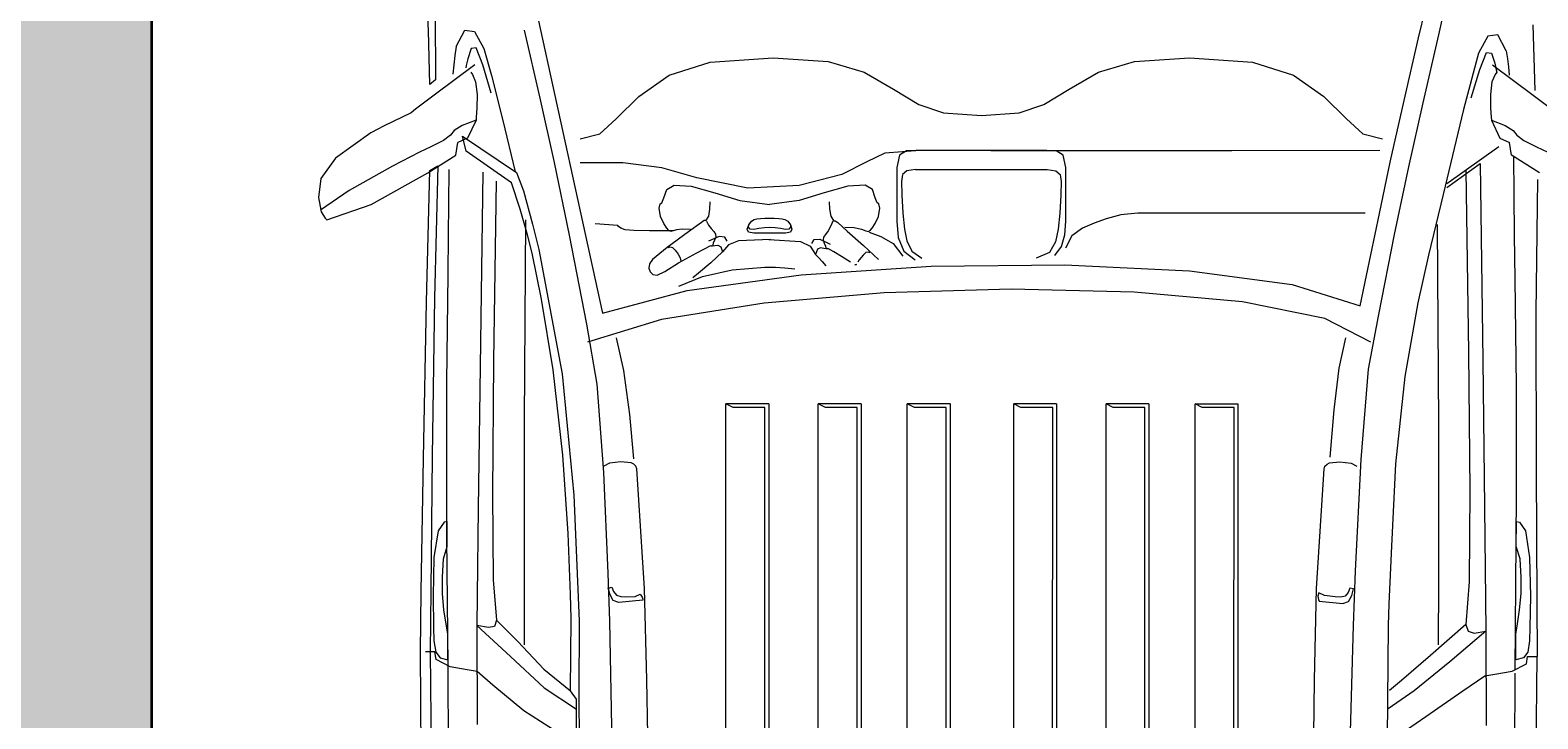
# Model space of a CAD drawing. Units: inches. Extents: x -16 to 587, y -783 to 64.
# Tile 4 of 14: x 111 to 195, y -633 to -595. Entities that reach past the tile are written whole.
import ezdxf

# ---------------------------------------------------------------- set-up
doc = ezdxf.new("R2010")
doc.units = ezdxf.units.IN
doc.header["$MEASUREMENT"] = 0
for name, color, linetype, lineweight in [('A-ANNO-DIMS', 2, 'Continuous', 18), ('A-SITE-VEHC', 8, 'Continuous', 13), ('A-WALL', 7, 'Continuous', 35), ('A-WALL-PATT', 23, 'Continuous', 13)]:
    doc.layers.add(name, color=color, linetype=linetype, lineweight=lineweight)
doc.styles.get("Standard").update_dxf_attribs({"font": 'arial.ttf'})
doc.dimstyles.get("Standard").update_dxf_attribs({"dimtxt": 0.18, "dimasz": 0.18, "dimexe": 0.18, "dimexo": 0.0625, "dimgap": 0.09, "dimtad": 0, "dimtih": 1, "dimtoh": 1, "dimdec": 0, "dimzin": 0, "dimdsep": 46, "dimlunit": 3, "dimtxsty": 'Standard', "dimcen": 0.09, "dimadec": 0, "dimazin": 0, "dimtfac": 1, "dimtdec": 0, "dimtofl": 0, "dimtmove": 0, "dimatfit": 3, "dimfxl": 1, "dimtolj": 1, "dimtzin": 0, "dimarcsym": 0})

# ---------------------------------------------------------------- blocks, each defined once
blk = doc.blocks.new('*D56')
at = {"layer": 'A-ANNO-DIMS', "color": 0, "lineweight": -2, "transparency": 16777216}
for p, q in [((118.083, -728.492), (118.083, 63.775)), ((228.083, -728.492), (228.083, 63.775)), ((118.263, 63.595), (172.753, 63.595)), ((227.903, 63.595), (173.412, 63.595))]:
    blk.add_line(p, q, dxfattribs=at)
at = {"layer": 'A-ANNO-DIMS', "color": 0, "transparency": 16777216}
for points in [[(118.263, 63.625), (118.263, 63.565), (118.083, 63.595)], [(227.903, 63.625), (227.903, 63.565), (228.083, 63.595)]]:
    blk.add_solid(points, dxfattribs=at)
at = {"layer": 'Defpoints', "color": 0, "transparency": 16777216}
for p in [(228.083, 63.595), (118.083, -728.555), (228.083, -728.555)]:
    blk.add_point(p, dxfattribs=at)
at = {"layer": 'A-ANNO-DIMS', "color": 0, "transparency": 16777216, "insert": (173.083, 63.595), "char_height": 0.18, "attachment_point": 5}
blk.add_mtext('\\A1;9\'-2"', dxfattribs=at)

msp = doc.modelspace()

# ---------------------------------------------------------------- hatches: boundary and pattern name
at = {"layer": 'A-WALL-PATT'}
h = msp.add_hatch(color=256, dxfattribs=at)
h.dxf.hatch_style = 1
h.paths.add_polyline_path([(137.083, -543.555), (137.083, -534.555), (118.083, -534.555), (118.083, -528.555), (109.083, -528.555), (109.083, -534.555), (109.083, -672.555), (118.083, -672.555), (118.083, -543.555)], flags=17)
h.paths.add_polyline_path([(27.083, -663.555), (27.083, -400.555), (73.083, -400.555), (73.083, -391.555), (27.083, -391.555), (27.083, 10.445), (48.751, 10.445), (171.083, 10.445), (171.083, -17.555), (180.083, -17.555), (180.083, 10.445), (228.083, 10.445), (228.083, -262.555), (206.414, -262.555), (118.083, -262.555), (118.083, -271.555), (228.083, -271.555), (228.083, -391.555), (154.083, -391.555), (154.083, -400.555), (228.083, -400.555), (228.083, -534.555), (209.083, -534.555), (209.083, -543.555), (237.083, -543.555), (237.083, 19.445), (18.083, 19.445), (18.083, -672.555), (73.083, -672.555), (73.083, -663.555)])
h.paths.add_polyline_path([(109.083, -486.555), (87.083, -486.555), (87.083, -495.555), (118.083, -495.555), (118.083, -400.555), (118.083, -391.555), (109.083, -391.555), (109.083, -400.555)], flags=17)

# ---------------------------------------------------------------- linework, layer by layer
at = {"layer": 'A-SITE-VEHC'}
for p, q in [((133.461, -595.126), (133.365, -593.07)), ((139.402, -593.833), (143.123, -610.827)), ((189.973, -593.605), (189.568, -595.361)), ((133.831, -594.204), (133.86, -597.859)), ((188.472, -595.539), (188.846, -593.942)), ((133.539, -598.134), (133.461, -595.126)), ((135.003, -596.012), (135.48, -595.11)), ((135.48, -595.11), (136.023, -595.18)), ((136.023, -595.18), (136.539, -596.13)), ((138.777, -595.108), (139.641, -598.886)), ((187.665, -599.023), (188.472, -595.539)), ((189.568, -595.361), (188.703, -599.139)), ((192.321, -595.433), (191.805, -596.383)), ((192.864, -595.363), (192.321, -595.433)), ((193.341, -596.265), (192.864, -595.363)), ((194.817, -594.806), (194.93, -598.464)), ((135.003, -596.012), (134.931, -596.516)), ((135.83, -596.13), (135.648, -596.695)), ((136.108, -596.091), (135.83, -596.13)), ((136.478, -597.036), (136.108, -596.091)), ((136.539, -596.13), (136.965, -597.635)), ((191.805, -596.383), (190.967, -599.517)), ((191.866, -597.289), (192.236, -596.343)), ((192.236, -596.343), (192.514, -596.383)), ((192.514, -596.383), (192.696, -596.948)), ((193.341, -596.265), (193.404, -596.702)), ((136.045, -597.033), (133.786, -598.721)), ((134.869, -597.03), (134.815, -597.554)), ((134.931, -596.516), (134.869, -597.03)), ((135.559, -597.063), (135.535, -597.194)), ((135.648, -596.695), (135.559, -597.063)), ((136.953, -598.612), (136.478, -597.036)), ((146.838, -597.613), (149.114, -596.892)), ((149.114, -596.892), (152.61, -596.647)), ((152.61, -596.647), (155.674, -596.854)), ((155.674, -596.854), (157.672, -597.445)), ((170.682, -597.445), (172.679, -596.854)), ((172.679, -596.854), (175.744, -596.647)), ((175.744, -596.647), (179.24, -596.892)), ((179.24, -596.892), (181.516, -597.613)), ((192.573, -597.033), (194.832, -598.721)), ((192.696, -596.948), (192.785, -597.315)), ((193.404, -596.702), (193.46, -597.147)), ((193.46, -597.147), (193.509, -597.6)), ((133.86, -597.859), (133.539, -598.134)), ((135.809, -597.447), (135.901, -597.571)), ((135.901, -597.571), (136.071, -597.972)), ((136.071, -597.972), (136.163, -598.688)), ((136.965, -597.635), (137.589, -600.122)), ((145.147, -598.791), (146.838, -597.613)), ((157.672, -597.445), (159.298, -598.38)), ((169.056, -598.38), (170.682, -597.445)), ((181.516, -597.613), (183.207, -598.791)), ((191.391, -598.865), (191.866, -597.289)), ((192.547, -597.972), (192.455, -598.688)), ((192.718, -597.571), (192.547, -597.972)), ((192.809, -597.447), (192.718, -597.571)), ((192.785, -597.315), (192.809, -597.447)), ((133.786, -598.721), (132.748, -599.502)), ((136.163, -598.688), (136.148, -599.449)), ((139.641, -598.886), (140.44, -602.454)), ((143.891, -600.03), (145.147, -598.791)), ((159.298, -598.38), (160.705, -599.245)), ((167.649, -599.245), (169.056, -598.38)), ((183.207, -598.791), (184.463, -600.03)), ((192.455, -598.688), (192.47, -599.449)), ((194.832, -598.721), (195.87, -599.502)), ((132.499, -599.693), (131.998, -599.935)), ((132.748, -599.502), (132.499, -599.693)), ((136.148, -599.449), (136.12, -599.935)), ((160.705, -599.245), (162.081, -599.704)), ((162.081, -599.704), (164.177, -599.84)), ((164.177, -599.84), (166.273, -599.704)), ((166.273, -599.704), (167.649, -599.245)), ((186.897, -602.432), (187.665, -599.023)), ((188.703, -599.139), (187.904, -602.707)), ((190.967, -599.517), (189.826, -604.241)), ((192.47, -599.449), (192.499, -599.935)), ((130.998, -600.427), (130.253, -600.815)), ((131.998, -599.935), (130.998, -600.427)), ((135.342, -600.4), (134.896, -600.68)), ((136.104, -600.106), (135.342, -600.4)), ((136.104, -600.106), (135.631, -601.111)), ((136.12, -599.935), (136.104, -600.106)), ((137.589, -600.122), (138.277, -602.975)), ((142.987, -600.86), (143.891, -600.03)), ((184.463, -600.03), (185.367, -600.86)), ((192.499, -599.935), (192.514, -600.106)), ((192.514, -600.106), (192.987, -601.111)), ((192.514, -600.106), (193.276, -600.4)), ((193.276, -600.4), (193.722, -600.68)), ((130.253, -600.815), (128.305, -602.219)), ((134.294, -601.231), (133.6, -601.582)), ((134.686, -600.934), (134.294, -601.231)), ((134.896, -600.68), (134.686, -600.934)), ((134.981, -602.057), (135.099, -601.347)), ((135.631, -601.111), (135.099, -601.347)), ((135.348, -600.995), (138.346, -603.01)), ((135.554, -601.82), (135.348, -600.995)), ((141.894, -601.147), (142.987, -600.86)), ((185.367, -600.86), (186.46, -601.147)), ((192.987, -601.111), (193.519, -601.347)), ((193.637, -602.057), (193.519, -601.347)), ((193.722, -600.68), (193.932, -600.934)), ((193.932, -600.934), (194.324, -601.231)), ((194.324, -601.231), (195.018, -601.582)), ((128.305, -602.219), (127.485, -603.354)), ((132.972, -601.879), (131.466, -602.664)), ((133.6, -601.582), (132.972, -601.879)), ((133.428, -603.026), (134.981, -602.057)), ((138.071, -603.582), (135.554, -601.82)), ((158.816, -601.944), (157.813, -602.417)), ((160.78, -601.785), (158.816, -601.944)), ((159.628, -602.053), (159.48, -602.729)), ((160.012, -601.816), (159.628, -602.053)), ((160.544, -601.787), (160.012, -601.816)), ((167.81, -601.787), (160.544, -601.787)), ((164.711, -601.806), (160.78, -601.785)), ((170.683, -601.818), (164.711, -601.806)), ((168.342, -601.816), (167.81, -601.787)), ((168.726, -602.053), (168.342, -601.816)), ((168.874, -602.729), (168.726, -602.053)), ((178.088, -601.817), (170.683, -601.818)), ((186.319, -601.797), (178.088, -601.817)), ((192.928, -601.584), (190.032, -603.652)), ((195.191, -603.026), (193.637, -602.057)), ((193.734, -602.087), (193.758, -604.239)), ((195.018, -601.582), (195.647, -601.879)), ((131.466, -602.664), (129.053, -604.01)), ((130.283, -604.792), (133.428, -603.026)), ((133.35, -610.198), (133.539, -602.896)), ((133.539, -602.896), (133.974, -602.635)), ((133.974, -602.635), (133.802, -609.976)), ((134.588, -602.844), (134.569, -604.738)), ((136.489, -602.992), (136.336, -613.783)), ((138.346, -603.01), (138.747, -604.031)), ((140.44, -602.454), (141.274, -606.488)), ((144.267, -602.483), (141.897, -602.483)), ((146.429, -602.758), (144.267, -602.483)), ((148.373, -603.308), (146.429, -602.758)), ((157.813, -602.417), (156.431, -603.124)), ((159.48, -602.729), (159.48, -605.709)), ((160.036, -602.913), (159.801, -603.119)), ((160.514, -602.851), (160.036, -602.913)), ((160.514, -602.851), (167.84, -602.851)), ((167.84, -602.851), (168.318, -602.913)), ((168.318, -602.913), (168.553, -603.119)), ((168.874, -605.709), (168.874, -602.729)), ((186.294, -605.289), (186.897, -602.432)), ((187.904, -602.707), (187.119, -606.463)), ((190.043, -603.856), (191.896, -602.516)), ((191.096, -602.884), (191.245, -613.003)), ((191.896, -602.516), (192.043, -613.432)), ((127.485, -603.354), (127.351, -604.401)), ((137.221, -603.495), (137.076, -613.478)), ((138.555, -605.059), (138.071, -603.582)), ((146.699, -603.954), (147.11, -603.714)), ((147.11, -603.714), (148.065, -603.778)), ((148.065, -603.778), (149.374, -604.147)), ((151.213, -603.879), (148.373, -603.308)), ((154.061, -603.741), (151.213, -603.879)), ((156.431, -603.124), (154.061, -603.741)), ((156.759, -603.778), (155.45, -604.147)), ((157.714, -603.714), (156.759, -603.778)), ((158.125, -603.954), (157.714, -603.714)), ((159.801, -603.119), (159.739, -603.505)), ((159.739, -603.505), (159.755, -604.255)), ((168.553, -603.119), (168.615, -603.505)), ((168.615, -603.505), (168.599, -604.255)), ((195.072, -603.399), (194.99, -610.784)), ((127.351, -604.401), (127.499, -605.196)), ((129.053, -604.01), (127.469, -605.111)), ((134.569, -604.738), (134.563, -606.509)), ((138.747, -604.031), (139.243, -605.888)), ((146.287, -604.995), (146.34, -604.757)), ((146.34, -604.757), (146.431, -604.705)), ((146.431, -604.705), (146.545, -604.417)), ((146.545, -604.417), (146.699, -603.954)), ((149.099, -604.645), (149.082, -605.054)), ((149.374, -604.147), (150.768, -604.576)), ((150.768, -604.576), (152.412, -604.782)), ((154.056, -604.576), (152.412, -604.782)), ((155.45, -604.147), (154.056, -604.576)), ((155.726, -604.645), (155.746, -605.052)), ((158.279, -604.417), (158.125, -603.954)), ((158.394, -604.705), (158.279, -604.417)), ((158.484, -604.757), (158.394, -604.705)), ((158.538, -604.995), (158.484, -604.757)), ((159.755, -604.255), (159.808, -605.272)), ((168.599, -604.255), (168.546, -605.272)), ((189.826, -604.241), (189.027, -607.612)), ((193.758, -604.239), (193.775, -606.514)), ((127.499, -605.196), (127.714, -605.557)), ((127.714, -605.557), (127.823, -605.642)), ((127.823, -605.642), (130.283, -604.792)), ((138.958, -606.485), (138.555, -605.059)), ((146.357, -605.451), (146.287, -604.995)), ((146.541, -605.84), (146.357, -605.451)), ((149.019, -605.446), (148.845, -605.705)), ((149.082, -605.054), (149.019, -605.446)), ((151.558, -605.623), (151.713, -605.587)), ((151.713, -605.587), (151.904, -605.562)), ((151.904, -605.562), (152.15, -605.547)), ((152.15, -605.547), (152.412, -605.542)), ((152.412, -605.542), (152.675, -605.547)), ((152.675, -605.547), (152.92, -605.562)), ((152.92, -605.562), (153.111, -605.587)), ((153.111, -605.587), (153.267, -605.623)), ((155.746, -605.052), (155.813, -605.443)), ((155.813, -605.443), (155.984, -605.709)), ((158.283, -605.84), (158.468, -605.451)), ((158.468, -605.451), (158.538, -604.995)), ((159.808, -605.272), (159.906, -606.165)), ((168.546, -605.272), (168.448, -606.165)), ((171.11, -605.581), (170.44, -605.825)), ((171.923, -605.368), (171.11, -605.581)), ((172.867, -605.276), (171.923, -605.368)), ((185.503, -605.276), (172.867, -605.276)), ((185.578, -608.743), (186.294, -605.289)), ((138.844, -605.646), (138.775, -616.807)), ((139.243, -605.888), (139.584, -607.295)), ((143.978, -605.963), (142.72, -605.871)), ((144.013, -606.012), (143.978, -605.963)), ((144.14, -606.112), (144.013, -606.012)), ((144.39, -606.192), (144.14, -606.112)), ((144.875, -606.229), (144.39, -606.192)), ((145.741, -606.249), (144.875, -606.229)), ((147.062, -606.256), (145.741, -606.249)), ((146.712, -606.104), (146.541, -605.84)), ((146.823, -606.238), (146.712, -606.104)), ((147.909, -606.314), (146.724, -607.187)), ((146.931, -606.284), (146.823, -606.238)), ((147.062, -606.256), (146.931, -606.284)), ((147.249, -606.196), (147.062, -606.256)), ((147.548, -606.159), (147.249, -606.196)), ((148.02, -606.18), (147.548, -606.159)), ((148.627, -605.785), (147.909, -606.314)), ((148.776, -605.688), (148.627, -605.785)), ((148.834, -605.688), (148.776, -605.688)), ((148.845, -605.705), (148.834, -605.688)), ((148.905, -605.708), (149.015, -605.941)), ((149.015, -605.941), (149.164, -606.128)), ((149.164, -606.128), (149.318, -606.291)), ((149.318, -606.291), (149.414, -606.446)), ((151.176, -606.168), (151.257, -605.922)), ((151.247, -606.323), (151.176, -606.168)), ((151.247, -606.046), (151.257, -605.922)), ((151.338, -606.157), (151.247, -606.046)), ((151.531, -606.377), (151.247, -606.323)), ((151.257, -605.922), (151.402, -605.713)), ((151.531, -606.18), (151.338, -606.157)), ((151.402, -605.713), (151.558, -605.623)), ((151.807, -606.132), (151.531, -606.18)), ((153.294, -606.377), (151.531, -606.377)), ((152.121, -606.091), (151.807, -606.132)), ((152.427, -606.074), (152.121, -606.091)), ((152.726, -606.091), (152.427, -606.074)), ((153.025, -606.132), (152.726, -606.091)), ((153.294, -606.18), (153.025, -606.132)), ((153.267, -605.623), (153.422, -605.713)), ((153.486, -606.157), (153.294, -606.18)), ((153.578, -606.323), (153.294, -606.377)), ((153.422, -605.713), (153.567, -605.922)), ((153.578, -606.046), (153.486, -606.157)), ((153.567, -605.922), (153.648, -606.168)), ((153.567, -605.922), (153.578, -606.046)), ((153.648, -606.168), (153.578, -606.323)), ((155.667, -606.251), (155.513, -606.454)), ((155.81, -605.983), (155.667, -606.251)), ((155.923, -605.709), (155.81, -605.983)), ((155.984, -605.709), (155.995, -605.692)), ((155.995, -605.692), (156.054, -605.695)), ((156.054, -605.695), (156.197, -605.8)), ((156.197, -605.8), (156.717, -606.263)), ((156.592, -606.059), (157.119, -606.069)), ((156.717, -606.263), (157.625, -607.075)), ((157.119, -606.069), (157.52, -606.164)), ((157.52, -606.164), (157.763, -606.256)), ((157.763, -606.256), (157.894, -606.284)), ((157.894, -606.284), (158.001, -606.238)), ((157.941, -606.329), (158.601, -606.572)), ((158.001, -606.238), (158.112, -606.104)), ((158.112, -606.104), (158.283, -605.84)), ((159.48, -605.709), (159.559, -606.629)), ((159.906, -606.165), (160.042, -606.804)), ((168.448, -606.165), (168.305, -606.866)), ((168.823, -606.471), (168.874, -605.709)), ((169.797, -606.101), (169.199, -606.534)), ((170.44, -605.825), (169.797, -606.101)), ((189.5, -605.898), (189.568, -616.994)), ((134.563, -606.509), (134.53, -608.66)), ((139.216, -607.497), (138.958, -606.485)), ((141.274, -606.488), (142.244, -611.446)), ((146.724, -607.187), (145.903, -607.848)), ((146.775, -607.178), (146.893, -607.145)), ((146.893, -607.145), (147.014, -607.184)), ((147.014, -607.184), (147.163, -607.335)), ((148.368, -607.47), (149.14, -607.074)), ((149.619, -606.566), (149.016, -606.824)), ((149.14, -607.074), (149.162, -607.081)), ((149.162, -607.081), (149.234, -607.087)), ((149.234, -607.087), (149.369, -607.07)), ((149.263, -607.034), (149.262, -607.065)), ((149.285, -606.94), (149.263, -607.034)), ((149.354, -606.78), (149.285, -606.94)), ((149.421, -606.603), (149.354, -606.78)), ((149.369, -607.07), (149.546, -607.051)), ((149.414, -606.446), (149.421, -606.603)), ((149.546, -607.051), (149.707, -607.136)), ((149.93, -606.608), (149.619, -606.566)), ((149.707, -607.136), (149.806, -607.428)), ((150.124, -607.026), (149.806, -607.428)), ((150.051, -606.832), (149.93, -606.608)), ((150.689, -606.808), (150.124, -607.026)), ((152.458, -606.743), (150.689, -606.808)), ((152.366, -606.743), (154.128, -606.837)), ((154.128, -606.837), (154.674, -607.114)), ((154.674, -607.114), (154.966, -607.563)), ((154.753, -606.955), (154.886, -606.737)), ((154.886, -606.737), (155.198, -606.712)), ((155.246, -607.201), (155.081, -607.277)), ((155.198, -606.712), (155.787, -607.001)), ((155.422, -607.229), (155.246, -607.201)), ((155.409, -606.603), (155.394, -606.76)), ((155.394, -606.76), (155.452, -606.94)), ((155.513, -606.454), (155.409, -606.603)), ((155.555, -607.253), (155.422, -607.229)), ((155.452, -606.94), (155.512, -607.103)), ((155.512, -607.103), (155.529, -607.198)), ((155.529, -607.198), (155.528, -607.229)), ((155.628, -607.25), (155.555, -607.253)), ((155.65, -607.244), (155.628, -607.25)), ((155.975, -607.425), (155.65, -607.244)), ((157.625, -607.075), (158.459, -607.843)), ((158.601, -606.572), (159.281, -606.956)), ((159.281, -606.956), (159.819, -607.657)), ((159.559, -606.629), (159.864, -607.376)), ((160.042, -606.804), (160.321, -607.389)), ((168.305, -606.866), (167.972, -607.457)), ((168.253, -607.625), (168.634, -607.125)), ((168.634, -607.125), (168.823, -606.471)), ((169.199, -606.534), (168.861, -607.222)), ((187.119, -606.463), (186.233, -610.904)), ((193.775, -606.514), (193.814, -608.912)), ((139.745, -610.054), (139.216, -607.497)), ((139.584, -607.295), (140.886, -614.201)), ((145.742, -608.088), (145.708, -608.319)), ((145.903, -607.848), (145.742, -608.088)), ((146.584, -608.507), (147.36, -608.03)), ((147.163, -607.335), (147.33, -607.552)), ((147.33, -607.552), (147.454, -607.756)), ((147.36, -608.03), (148.368, -607.47)), ((147.454, -607.756), (147.481, -607.946)), ((149.15, -608.027), (148.47, -608.609)), ((149.806, -607.428), (149.15, -608.027)), ((155.081, -607.277), (154.966, -607.563)), ((154.966, -607.563), (155.144, -607.759)), ((155.144, -607.759), (155.327, -607.96)), ((155.327, -607.96), (155.545, -608.197)), ((156.407, -607.681), (155.975, -607.425)), ((156.913, -607.993), (156.407, -607.681)), ((157.391, -607.868), (157.31, -607.991)), ((157.496, -607.74), (157.391, -607.868)), ((157.611, -607.609), (157.496, -607.74)), ((157.767, -607.465), (157.611, -607.609)), ((157.89, -607.433), (157.767, -607.465)), ((158.006, -607.472), (157.89, -607.433)), ((159.864, -607.376), (160.493, -607.87)), ((160.321, -607.389), (160.875, -607.775)), ((167.972, -607.457), (167.231, -607.763)), ((189.027, -607.612), (188.434, -610.261)), ((134.53, -608.66), (134.462, -614.651)), ((145.708, -608.319), (145.776, -608.526)), ((145.776, -608.526), (145.923, -608.684)), ((145.923, -608.684), (146.175, -608.711)), ((146.175, -608.711), (146.584, -608.507)), ((147.369, -609.318), (148.694, -608.791)), ((147.836, -609.57), (154.159, -608.696)), ((148.47, -608.609), (148.156, -608.87)), ((148.694, -608.791), (150.332, -608.419)), ((150.332, -608.419), (152.154, -608.277)), ((152.154, -608.277), (152.742, -608.279)), ((152.742, -608.279), (153.263, -608.301)), ((153.263, -608.301), (153.809, -608.364)), ((154.159, -608.696), (161.388, -608.216)), ((157.155, -608.137), (157.241, -608.131)), ((157.184, -608.135), (157.155, -608.137)), ((157.212, -608.133), (157.184, -608.135)), ((157.241, -608.131), (157.212, -608.133)), ((161.388, -608.216), (168.815, -608.138)), ((168.815, -608.138), (175.736, -608.474)), ((175.736, -608.474), (181.444, -609.231)), ((185.232, -610.422), (185.578, -608.743)), ((193.814, -608.912), (193.882, -614.904)), ((143.123, -610.827), (147.836, -609.57)), ((158.78, -609.698), (152.103, -610.262)), ((165.837, -609.493), (158.78, -609.698)), ((172.671, -609.656), (165.837, -609.493)), ((178.679, -610.195), (172.671, -609.656)), ((181.444, -609.231), (185.232, -610.422)), ((133.182, -618.895), (133.35, -610.198)), ((133.802, -609.976), (133.674, -618.763)), ((140.381, -613.966), (139.745, -610.054)), ((152.103, -610.262), (146.406, -611.178)), ((183.261, -611.119), (178.679, -610.195)), ((188.434, -610.261), (187.709, -614.341)), ((142.244, -611.446), (142.821, -614.763)), ((146.406, -611.178), (142.292, -612.436)), ((185.814, -612.436), (183.261, -611.119)), ((186.233, -610.904), (185.674, -613.939)), ((194.99, -610.784), (194.993, -619.531)), ((143.886, -612.19), (144.288, -614.006)), ((184.415, -612.19), (184.044, -613.89)), ((191.245, -613.003), (191.317, -620.666)), ((136.336, -613.783), (136.23, -621.675)), ((137.076, -613.478), (137.013, -620.845)), ((140.933, -618.714), (140.381, -613.966)), ((184.044, -613.89), (183.753, -616.196)), ((185.674, -613.939), (185.253, -618.945)), ((192.043, -613.432), (192.137, -621.599)), ((134.462, -614.651), (134.46, -620.576)), ((140.886, -614.201), (141.54, -620.929)), ((142.821, -614.763), (143.188, -619.684)), ((144.288, -614.006), (144.629, -616.447)), ((187.709, -614.341), (187.195, -619.196)), ((193.882, -614.904), (193.884, -620.829)), ((144.629, -616.447), (144.848, -618.919)), ((150.391, -616.064), (149.987, -615.867)), ((152.369, -615.867), (149.987, -615.867)), ((149.989, -678.315), (149.989, -615.867)), ((152.153, -616.064), (150.391, -616.064)), ((152.131, -677.322), (152.153, -616.064)), ((152.368, -615.867), (152.368, -678.315)), ((152.369, -615.867), (152.369, -678.315)), ((155.519, -616.064), (155.114, -615.867)), ((157.497, -615.867), (155.114, -615.867)), ((155.117, -678.315), (155.117, -615.867)), ((157.281, -616.064), (155.519, -616.064)), ((157.258, -677.322), (157.281, -616.064)), ((157.495, -615.867), (157.495, -678.315)), ((157.497, -615.867), (157.497, -678.315)), ((160.463, -616.064), (160.059, -615.867)), ((162.442, -615.867), (160.059, -615.867)), ((160.061, -678.315), (160.061, -615.867)), ((162.226, -616.064), (160.463, -616.064)), ((162.203, -677.322), (162.226, -616.064)), ((162.44, -615.867), (162.44, -678.315)), ((162.442, -615.867), (162.442, -678.315)), ((166.379, -616.064), (165.975, -615.867)), ((168.358, -615.867), (165.975, -615.867)), ((165.977, -678.315), (165.977, -615.867)), ((168.142, -616.064), (166.379, -616.064)), ((168.119, -677.322), (168.142, -616.064)), ((168.355, -615.867), (168.355, -678.315)), ((168.358, -615.867), (168.358, -678.315)), ((171.507, -616.064), (171.103, -615.867)), ((173.485, -615.867), (171.103, -615.867)), ((171.105, -678.315), (171.105, -615.867)), ((173.269, -616.064), (171.507, -616.064)), ((173.247, -677.322), (173.269, -616.064)), ((173.483, -615.867), (173.483, -678.315)), ((173.485, -615.867), (173.485, -678.315)), ((176.049, -678.315), (176.049, -615.867)), ((176.453, -616.064), (176.049, -615.867)), ((176.049, -615.867), (178.43, -615.867)), ((178.216, -616.064), (176.453, -616.064)), ((178.193, -677.322), (178.216, -616.064)), ((178.43, -615.867), (178.43, -678.315)), ((183.753, -616.196), (183.535, -618.828)), ((138.775, -616.807), (138.771, -625.648)), ((189.568, -616.994), (189.57, -625.713)), ((133.062, -626.276), (133.182, -618.895)), ((133.674, -618.763), (133.593, -626.234)), ((141.23, -623.061), (140.933, -618.714)), ((185.253, -618.945), (184.948, -625.145)), ((143.188, -619.684), (143.428, -625.268)), ((143.525, -619.149), (143.198, -619.332)), ((144.151, -619.08), (143.525, -619.149)), ((144.717, -619.135), (144.151, -619.08)), ((144.862, -619.207), (144.717, -619.135)), ((144.979, -619.325), (144.862, -619.207)), ((145.031, -619.469), (144.979, -619.325)), ((145.459, -626.126), (145.031, -619.469)), ((182.8, -626.126), (183.214, -619.469)), ((183.214, -619.469), (183.266, -619.325)), ((183.266, -619.325), (183.383, -619.207)), ((183.383, -619.207), (183.528, -619.135)), ((183.528, -619.135), (184.093, -619.08)), ((184.093, -619.08), (184.719, -619.149)), ((184.719, -619.149), (185.047, -619.332)), ((187.195, -619.196), (186.956, -623.758)), ((194.993, -619.531), (195.031, -626.836)), ((134.46, -620.576), (134.471, -623.258)), ((191.317, -620.666), (191.279, -625.748)), ((137.013, -620.845), (137.061, -625.63)), ((141.54, -620.929), (141.838, -627.921)), ((193.884, -620.829), (193.874, -623.511)), ((136.23, -621.675), (136.169, -626.52)), ((192.137, -621.599), (192.186, -626.72)), ((133.996, -622.912), (133.764, -624.399)), ((134.326, -622.434), (133.996, -622.912)), ((134.494, -622.4), (134.326, -622.434)), ((134.508, -623.794), (134.494, -622.4)), ((141.361, -626.427), (141.23, -623.061)), ((193.894, -623.794), (193.907, -622.4)), ((193.907, -622.4), (194.075, -622.434)), ((194.075, -622.434), (194.405, -622.912)), ((194.405, -622.912), (194.637, -624.399)), ((134.297, -624.479), (134.508, -623.794)), ((134.471, -623.258), (134.53, -630.409)), ((186.956, -623.758), (186.823, -626.967)), ((193.874, -623.511), (193.814, -630.662)), ((194.104, -624.479), (193.894, -623.794)), ((133.764, -624.399), (133.724, -626.535)), ((134.24, -625.489), (134.297, -624.479)), ((194.161, -625.489), (194.104, -624.479)), ((194.637, -624.399), (194.678, -626.535)), ((134.242, -626.399), (134.24, -625.489)), ((137.061, -625.63), (137.248, -627.868)), ((138.771, -625.648), (138.781, -629.244)), ((143.428, -625.268), (143.513, -627.927)), ((184.948, -625.145), (184.831, -628.18)), ((194.16, -626.399), (194.161, -625.489)), ((133.014, -629.627), (133.062, -626.276)), ((133.593, -626.234), (133.563, -629.627)), ((133.724, -626.535), (133.747, -628.289)), ((134.319, -627.298), (134.242, -626.399)), ((136.169, -626.52), (136.149, -628.168)), ((141.391, -627.779), (141.361, -626.427)), ((143.451, -626.093), (143.656, -626.051)), ((143.547, -626.469), (143.451, -626.093)), ((143.722, -626.788), (143.547, -626.469)), ((143.656, -626.051), (143.742, -626.293)), ((143.742, -626.293), (143.906, -626.496)), ((143.906, -626.496), (144.149, -626.562)), ((144.952, -626.563), (145.227, -626.441)), ((145.227, -626.441), (145.331, -626.595)), ((145.592, -631.197), (145.459, -626.126)), ((182.694, -631.197), (182.8, -626.126)), ((182.936, -626.35), (182.868, -626.539)), ((183.247, -626.507), (182.936, -626.35)), ((183.834, -626.586), (183.247, -626.507)), ((184.559, -626.339), (184.395, -626.541)), ((184.645, -626.096), (184.559, -626.339)), ((184.579, -626.834), (184.754, -626.515)), ((184.849, -626.139), (184.645, -626.096)), ((184.754, -626.515), (184.849, -626.139)), ((189.57, -625.713), (189.559, -629.244)), ((191.279, -625.748), (191.096, -628.121)), ((194.083, -627.298), (194.16, -626.399)), ((194.678, -626.535), (194.655, -628.289)), ((134.462, -628.216), (134.319, -627.298)), ((144.033, -626.9), (143.722, -626.788)), ((145.362, -626.769), (144.033, -626.9)), ((144.149, -626.562), (144.431, -626.576)), ((144.431, -626.576), (144.952, -626.563)), ((145.331, -626.595), (145.362, -626.719)), ((145.362, -626.719), (145.362, -626.769)), ((182.868, -626.539), (182.903, -626.729)), ((182.903, -626.729), (182.938, -626.815)), ((182.938, -626.815), (184.268, -626.946)), ((184.151, -626.607), (183.834, -626.586)), ((184.395, -626.541), (184.151, -626.607)), ((184.268, -626.946), (184.579, -626.834)), ((186.823, -626.967), (186.781, -628.18)), ((192.186, -626.72), (192.201, -628.493)), ((193.94, -628.216), (194.083, -627.298)), ((195.031, -626.836), (195.055, -629.894)), ((136.149, -628.168), (138.013, -629.893)), ((136.788, -628.287), (136.149, -628.168)), ((136.149, -628.168), (136.172, -633.662)), ((137.248, -627.868), (137.121, -628.221)), ((137.248, -627.868), (138.433, -629.053)), ((141.356, -631.803), (141.391, -627.779)), ((141.838, -627.921), (141.81, -632.032)), ((143.513, -627.927), (143.651, -634.79)), ((184.831, -628.18), (184.658, -634.742)), ((186.781, -628.18), (186.726, -634.447)), ((191.096, -628.121), (189.136, -629.845)), ((191.096, -628.121), (191.224, -628.493)), ((133.747, -628.289), (133.768, -629.017)), ((133.768, -629.017), (133.862, -629.657)), ((134.538, -628.637), (134.462, -628.216)), ((134.538, -630.087), (134.538, -628.637)), ((137.121, -628.221), (136.788, -628.287)), ((192.201, -628.493), (190.206, -630.185)), ((191.224, -628.493), (191.559, -628.593)), ((191.559, -628.593), (192.201, -628.493)), ((192.201, -628.493), (192.219, -633.733)), ((193.863, -628.637), (193.94, -628.216)), ((193.863, -630.087), (193.863, -628.637)), ((194.633, -629.017), (194.54, -629.657)), ((194.655, -628.289), (194.633, -629.017)), ((133.062, -635.266), (133.014, -629.627)), ((133.82, -629.641), (133.289, -629.627)), ((133.563, -629.627), (133.612, -635.26)), ((133.88, -630.055), (133.82, -629.641)), ((133.862, -629.657), (134.109, -629.972)), ((138.433, -629.053), (139.874, -630.607)), ((189.136, -629.845), (187.518, -631.224)), ((194.54, -629.657), (194.293, -629.972)), ((134.671, -630.467), (133.88, -630.055)), ((134.109, -629.972), (134.538, -630.087)), ((134.53, -630.409), (134.576, -639.048)), ((135.617, -630.635), (134.671, -630.467)), ((136.172, -630.732), (135.617, -630.635)), ((138.013, -629.893), (139.886, -631.626)), ((139.874, -630.607), (141.356, -631.803)), ((190.206, -630.185), (188.228, -631.809)), ((192.705, -630.87), (193.665, -630.713)), ((193.665, -630.713), (194.464, -630.307)), ((194.293, -629.972), (193.863, -630.087)), ((194.464, -630.307), (194.524, -629.894)), ((194.524, -629.894), (195.034, -629.894)), ((195.007, -635.526), (195.055, -629.894)), ((137.034, -631.486), (136.172, -630.732)), ((138.765, -632.909), (137.034, -631.486)), ((145.651, -634.256), (145.592, -631.197)), ((182.649, -634.256), (182.694, -631.197)), ((187.518, -631.224), (186.844, -631.787)), ((190.935, -631.795), (192.142, -630.961)), ((192.142, -630.961), (192.705, -630.87)), ((193.822, -630.822), (193.776, -639.461)), ((139.886, -631.626), (141.688, -632.815)), ((141.678, -632.257), (141.356, -631.803)), ((141.7, -636.249), (141.678, -632.257)), ((141.81, -632.032), (141.839, -634.647)), ((188.228, -631.809), (186.785, -632.792)), ((188.879, -633.219), (190.935, -631.795)), ((140.613, -634.097), (138.765, -632.909)), ((187.79, -633.974), (188.879, -633.219))]:
    msp.add_line(p, q, dxfattribs=at)
at = {"layer": 'A-WALL'}
msp.add_line((118.083, -543.555), (118.083, -672.555), dxfattribs=at)

# ---------------------------------------------------------------- dimensions: what is measured, and where the dimension line sits
at = {"layer": 'A-ANNO-DIMS'}
dim = msp.add_linear_dim(base=(228.083, 63.595), p1=(118.083, -728.555), p2=(228.083, -728.555), dimstyle='Standard', override={"dimdec": 1, "dimlfac": 1, "dimrnd": 0, "dimzin": 1, "dimdsep": 46, "dimlunit": 4, "dimfrac": 2}, dxfattribs=at)
dim.commit()
dim.dimension.update_dxf_attribs({"geometry": '*D56', "text_midpoint": (173.083, 63.595)})

doc.saveas('drawing.dxf')
